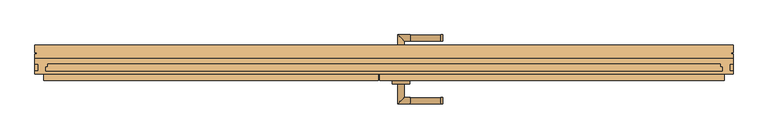
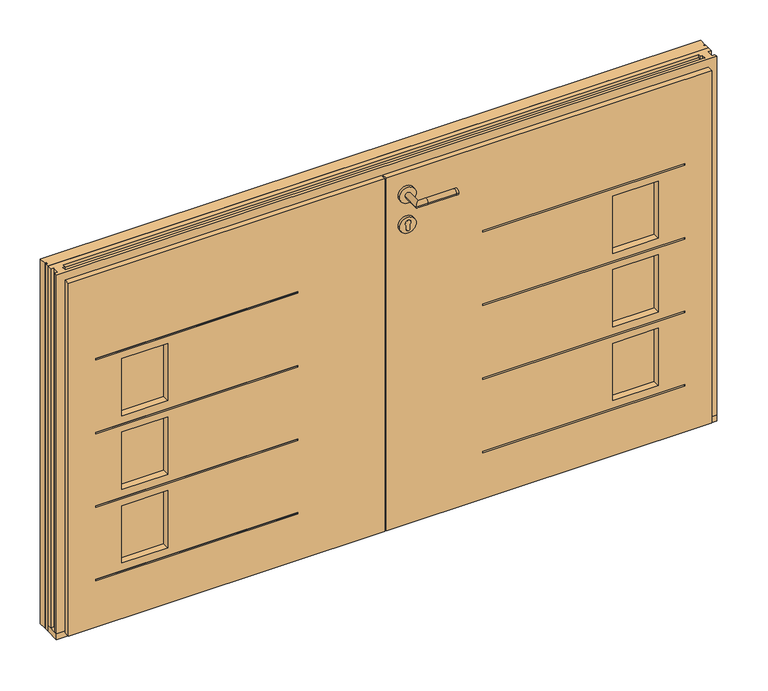
"""IFC4 building model written with IfcOpenShell, lengths in millimetres: door geometry."""

from ifc_helpers import new_model, si_unit, point, frame, frame_2d, origin, origin_with_axes, place, context, project, spatial, polyline, circle_curve, ellipse_curve, trimmed, segment, composite_curve, outline, extrude, faceted_brep, source, transform, mapped, element, save
from ifc_brep_helpers import plane_surface, cylinder_surface, advanced_brep


def door_97be9440(model_context):
    return source(origin(), model_context, "Body", "SolidModel", [
        extrude(outline(polyline([(922.0, -28.0), (922.0, -56.0), (82.0, -56.0), (82.0, -28.0), (922.0, -28.0)])), frame((0.0, 0.0, 108.0), z_axis=(0.0, 0.0, 1.0), x_axis=(1.0, 0.0, 0.0)), (0.0, 0.0, 1.0), 990.2),
        advanced_brep(
        [(60.1308541, -89.0, 1120.0), (41.1308541, -89.0, 1120.0), (41.1308541, -149.0, 1120.0), (60.1308541, -130.0, 1120.0), (176.1308541, -130.0, 1120.0), (176.1308541, -149.0, 1120.0), (170.1308541, -130.0, 1120.0), (170.1308541, -149.0, 1120.0), (79.1308541, -149.0, 1120.0), (79.1308541, -130.0, 1120.0), (170.1308541, -130.5, 1120.0), (170.1308541, -148.5, 1120.0), (79.1308541, -130.5, 1120.0), (79.1308541, -148.5, 1120.0)],
        [
            (0, 1, circle_curve(frame((50.6308541, -89.0, 1120.0), z_axis=(0.0, 1.0, 0.0), x_axis=(-1.0, 0.0, 0.0)), 9.5)),
            (1, 0, circle_curve(frame((50.6308541, -89.0, 1120.0), z_axis=(0.0, 1.0, 0.0), x_axis=(-1.0, 0.0, 0.0)), 9.5)),
            (1, 2),
            (2, 3, ellipse_curve(frame((50.6308541, -139.5, 1120.0), z_axis=(-0.7071067811865475, 0.7071067811865475, 0.0), x_axis=(0.7071067811865474, 0.7071067811865476, 0.0)), 13.4350288, 9.5)),
            (3, 0),
            (3, 2, ellipse_curve(frame((50.6308541, -139.5, 1120.0), z_axis=(-0.7071067811865475, 0.7071067811865475, 0.0), x_axis=(0.7071067811865474, 0.7071067811865476, 0.0)), 13.4350288, 9.5)),
            (4, 5, circle_curve(frame((176.1308541, -139.5, 1120.0), z_axis=(1.0, 0.0, 0.0), x_axis=(0.0, -1.0, 0.0)), 9.5)),
            (5, 4, circle_curve(frame((176.1308541, -139.5, 1120.0), z_axis=(1.0, 0.0, 0.0), x_axis=(0.0, -1.0, 0.0)), 9.5)),
            (4, 6),
            (6, 7, circle_curve(frame((170.1308541, -139.5, 1120.0), z_axis=(1.0, 0.0, 0.0), x_axis=(0.0, -1.0, 0.0)), 9.5)),
            (7, 5),
            (2, 8),
            (8, 9, circle_curve(frame((79.1308541, -139.5, 1120.0), z_axis=(-1.0, 0.0, 0.0), x_axis=(0.0, -1.0, 0.0)), 9.5)),
            (9, 3),
            (9, 8, circle_curve(frame((79.1308541, -139.5, 1120.0), z_axis=(-1.0, 0.0, 0.0), x_axis=(0.0, -1.0, 0.0)), 9.5)),
            (7, 6, circle_curve(frame((170.1308541, -139.5, 1120.0), z_axis=(1.0, 0.0, 0.0), x_axis=(0.0, -1.0, 0.0)), 9.5)),
            (10, 11, circle_curve(frame((170.1308541, -139.5, 1120.0), z_axis=(1.0, 0.0, 0.0), x_axis=(0.0, -1.0, 0.0)), 9.0)),
            (11, 10, circle_curve(frame((170.1308541, -139.5, 1120.0), z_axis=(1.0, 0.0, 0.0), x_axis=(0.0, -1.0, 0.0)), 9.0)),
            (12, 13, circle_curve(frame((79.1308541, -139.5, 1120.0), z_axis=(-1.0, 0.0, 0.0), x_axis=(0.0, -1.0, 0.0)), 9.0)),
            (13, 12, circle_curve(frame((79.1308541, -139.5, 1120.0), z_axis=(-1.0, 0.0, 0.0), x_axis=(0.0, -1.0, 0.0)), 9.0)),
            (10, 12),
            (13, 11),
        ],
        [
            plane_surface(frame((50.6308541, -89.0, 1120.0), z_axis=(0.0, 1.0, 0.0), x_axis=(0.0, 0.0, 1.0))),
            cylinder_surface(frame((50.6308541, -89.0, 1120.0), z_axis=(0.0, 1.0, 0.0), x_axis=(-1.0, 0.0, 0.0)), 9.5),
            plane_surface(frame((176.1308541, -139.5, 1120.0), z_axis=(1.0, 0.0, 0.0), x_axis=(0.0, 0.0, 1.0))),
            cylinder_surface(frame((50.6308541, -139.5, 1120.0), z_axis=(-1.0, 0.0, 0.0), x_axis=(0.0, -1.0, 0.0)), 9.5),
            plane_surface(frame((170.1308541, -149.0, 1120.0), z_axis=(-1.0, 0.0, 0.0), x_axis=(0.0, 0.0, 1.0))),
            plane_surface(frame((79.1308541, -149.0, 1120.0), z_axis=(1.0, 0.0, 0.0), x_axis=(0.0, 0.0, -1.0))),
            cylinder_surface(frame((50.6308541, -139.5, 1120.0), z_axis=(-1.0, 0.0, 0.0), x_axis=(0.0, -1.0, 0.0)), 9.0),
        ],
        [
            (0, [[1, 2]]),
            (1, [[3, 4, 5, -2]]),
            (1, [[-5, 6, -3, -1]]),
            (2, [[7, 8]]),
            (3, [[9, 10, 11, -7]]),
            (3, [[12, 13, 14, -4]]),
            (3, [[-14, 15, -12, -6]]),
            (3, [[-11, 16, -9, -8]]),
            (4, [[-16, -10], [17, 18]]),
            (5, [[-15, -13], [19, 20]]),
            (6, [[21, -20, 22, -17]]),
            (6, [[-22, -19, -21, -18]]),
        ],
    ),
        extrude(outline(composite_curve([segment(trimmed(circle_curve(frame_2d((1019.75, 50.6308541)), 26.0), [point((1019.75, 24.6308541))], [point((1019.75, 76.6308541))], False, "CARTESIAN"), True, "CONTINUOUS"), segment(trimmed(circle_curve(frame_2d((1019.75, 50.6308541)), 26.0), [point((1019.75, 76.6308541))], [point((1019.75, 24.6308541))], False, "CARTESIAN"), True, "CONTINUOUS")], self_intersect=False)), frame((0.0, -89.0, 0.0), z_axis=(0.0, 1.0, 0.0), x_axis=(0.0, 0.0, 1.0)), (0.0, 0.0, 1.0), 10.0),
        extrude(outline(composite_curve([segment(polyline([(1021.404547, 44.8808541), (1008.0, 44.8808541)]), True, "CONTINUOUS"), segment(trimmed(circle_curve(frame_2d((1008.0, 50.6308541)), 5.75), [point((1008.0, 44.8808541))], [point((1008.0, 56.3808541))], False, "CARTESIAN"), True, "CONTINUOUS"), segment(polyline([(1008.0, 56.3808541), (1021.404547, 56.3808541)]), True, "CONTINUOUS"), segment(trimmed(circle_curve(frame_2d((1028.0, 50.6308541)), 8.75), [point((1021.404547, 56.3808541))], [point((1021.404547, 44.8808541))], False, "CARTESIAN"), True, "CONTINUOUS")], self_intersect=False)), frame((0.0, -90.0, 0.0), z_axis=(0.0, 1.0, 0.0), x_axis=(0.0, 0.0, 1.0)), (0.0, 0.0, 1.0), 1.0),
        extrude(outline(composite_curve([segment(trimmed(circle_curve(frame_2d((1120.0, 50.6308541)), 26.0), [point((1120.0, 24.6308541))], [point((1120.0, 76.6308541))], False, "CARTESIAN"), True, "CONTINUOUS"), segment(trimmed(circle_curve(frame_2d((1120.0, 50.6308541)), 26.0), [point((1120.0, 76.6308541))], [point((1120.0, 24.6308541))], False, "CARTESIAN"), True, "CONTINUOUS")], self_intersect=False)), frame((0.0, -89.0, 0.0), z_axis=(0.0, 1.0, 0.0), x_axis=(0.0, 0.0, 1.0)), (0.0, 0.0, 1.0), 10.0),
        advanced_brep(
        [(60.1308541, -2.0, 1120.0), (41.1308541, -2.0, 1120.0), (60.1308541, 39.0, 1120.0), (41.1308541, 58.0, 1120.0), (176.1308541, 39.0, 1120.0), (176.1308541, 58.0, 1120.0), (79.1308541, 39.0, 1120.0), (79.1308541, 58.0, 1120.0), (170.1308541, 58.0, 1120.0), (170.1308541, 39.0, 1120.0), (170.1308541, 39.5, 1120.0), (170.1308541, 57.5, 1120.0), (79.1308541, 39.5, 1120.0), (79.1308541, 57.5, 1120.0)],
        [
            (0, 1, circle_curve(frame((50.6308541, -2.0, 1120.0), z_axis=(0.0, -1.0, 0.0), x_axis=(-1.0, 0.0, 0.0)), 9.5)),
            (1, 0, circle_curve(frame((50.6308541, -2.0, 1120.0), z_axis=(0.0, -1.0, 0.0), x_axis=(-1.0, 0.0, 0.0)), 9.5)),
            (0, 2),
            (2, 3, ellipse_curve(frame((50.6308541, 48.5, 1120.0), z_axis=(-0.7071067811865475, -0.7071067811865475, 0.0), x_axis=(0.7071067811865474, -0.7071067811865476, 0.0)), 13.4350288, 9.5)),
            (3, 1),
            (3, 2, ellipse_curve(frame((50.6308541, 48.5, 1120.0), z_axis=(-0.7071067811865475, -0.7071067811865475, 0.0), x_axis=(0.7071067811865474, -0.7071067811865476, 0.0)), 13.4350288, 9.5)),
            (4, 5, circle_curve(frame((176.1308541, 48.5, 1120.0), z_axis=(1.0, 0.0, 0.0), x_axis=(0.0, 1.0, 0.0)), 9.5)),
            (5, 4, circle_curve(frame((176.1308541, 48.5, 1120.0), z_axis=(1.0, 0.0, 0.0), x_axis=(0.0, 1.0, 0.0)), 9.5)),
            (2, 6),
            (6, 7, circle_curve(frame((79.1308541, 48.5, 1120.0), z_axis=(-1.0, 0.0, 0.0), x_axis=(0.0, 1.0, 0.0)), 9.5)),
            (7, 3),
            (5, 8),
            (8, 9, circle_curve(frame((170.1308541, 48.5, 1120.0), z_axis=(1.0, 0.0, 0.0), x_axis=(0.0, 1.0, 0.0)), 9.5)),
            (9, 4),
            (7, 6, circle_curve(frame((79.1308541, 48.5, 1120.0), z_axis=(-1.0, 0.0, 0.0), x_axis=(0.0, 1.0, 0.0)), 9.5)),
            (9, 8, circle_curve(frame((170.1308541, 48.5, 1120.0), z_axis=(1.0, 0.0, 0.0), x_axis=(0.0, 1.0, 0.0)), 9.5)),
            (10, 11, circle_curve(frame((170.1308541, 48.5, 1120.0), z_axis=(1.0, 0.0, 0.0), x_axis=(0.0, 1.0, 0.0)), 9.0)),
            (11, 10, circle_curve(frame((170.1308541, 48.5, 1120.0), z_axis=(1.0, 0.0, 0.0), x_axis=(0.0, 1.0, 0.0)), 9.0)),
            (12, 13, circle_curve(frame((79.1308541, 48.5, 1120.0), z_axis=(-1.0, 0.0, 0.0), x_axis=(0.0, 1.0, 0.0)), 9.0)),
            (13, 12, circle_curve(frame((79.1308541, 48.5, 1120.0), z_axis=(-1.0, 0.0, 0.0), x_axis=(0.0, 1.0, 0.0)), 9.0)),
            (11, 13),
            (12, 10),
        ],
        [
            plane_surface(frame((50.6308541, -2.0, 1120.0), z_axis=(0.0, -1.0, 0.0), x_axis=(0.0, 0.0, 1.0))),
            cylinder_surface(frame((50.6308541, -2.0, 1120.0), z_axis=(0.0, -1.0, 0.0), x_axis=(-1.0, 0.0, 0.0)), 9.5),
            plane_surface(frame((176.1308541, 48.5, 1120.0), z_axis=(1.0, 0.0, 0.0), x_axis=(0.0, 0.0, 1.0))),
            cylinder_surface(frame((50.6308541, 48.5, 1120.0), z_axis=(-1.0, 0.0, 0.0), x_axis=(0.0, 1.0, 0.0)), 9.5),
            plane_surface(frame((170.1308541, 58.0, 1120.0), z_axis=(-1.0, 0.0, 0.0), x_axis=(0.0, 0.0, 1.0))),
            plane_surface(frame((79.1308541, 58.0, 1120.0), z_axis=(1.0, 0.0, 0.0), x_axis=(0.0, 0.0, -1.0))),
            cylinder_surface(frame((50.6308541, 48.5, 1120.0), z_axis=(-1.0, 0.0, 0.0), x_axis=(0.0, 1.0, 0.0)), 9.0),
        ],
        [
            (0, [[1, 2]]),
            (1, [[-1, 3, 4, 5]]),
            (1, [[-2, -5, 6, -3]]),
            (2, [[7, 8]]),
            (3, [[-4, 9, 10, 11]]),
            (3, [[-8, 12, 13, 14]]),
            (3, [[-6, -11, 15, -9]]),
            (3, [[-7, -14, 16, -12]]),
            (4, [[-13, -16], [17, 18]]),
            (5, [[-10, -15], [19, 20]]),
            (6, [[-18, 21, -19, 22]]),
            (6, [[-17, -22, -20, -21]]),
        ],
    ),
        extrude(outline(composite_curve([segment(trimmed(circle_curve(frame_2d((1019.75, 50.6308541)), 26.0), [point((1019.75, 24.6308541))], [point((1019.75, 76.6308541))], False, "CARTESIAN"), True, "CONTINUOUS"), segment(trimmed(circle_curve(frame_2d((1019.75, 50.6308541)), 26.0), [point((1019.75, 76.6308541))], [point((1019.75, 24.6308541))], False, "CARTESIAN"), True, "CONTINUOUS")], self_intersect=False)), frame((0.0, -12.0, 0.0), z_axis=(0.0, 1.0, 0.0), x_axis=(0.0, 0.0, 1.0)), (0.0, 0.0, 1.0), 10.0),
        extrude(outline(composite_curve([segment(polyline([(1021.404547, 44.8808541), (1008.0, 44.8808541)]), True, "CONTINUOUS"), segment(trimmed(circle_curve(frame_2d((1008.0, 50.6308541)), 5.75), [point((1008.0, 44.8808541))], [point((1008.0, 56.3808541))], False, "CARTESIAN"), True, "CONTINUOUS"), segment(polyline([(1008.0, 56.3808541), (1021.404547, 56.3808541)]), True, "CONTINUOUS"), segment(trimmed(circle_curve(frame_2d((1028.0, 50.6308541)), 8.75), [point((1021.404547, 56.3808541))], [point((1021.404547, 44.8808541))], False, "CARTESIAN"), True, "CONTINUOUS")], self_intersect=False)), frame((0.0, -2.0, 0.0), z_axis=(0.0, 1.0, 0.0), x_axis=(0.0, 0.0, 1.0)), (0.0, 0.0, 1.0), 1.0),
        extrude(outline(composite_curve([segment(trimmed(circle_curve(frame_2d((1120.0, 50.6308541)), 26.0), [point((1120.0, 24.6308541))], [point((1120.0, 76.6308541))], False, "CARTESIAN"), True, "CONTINUOUS"), segment(trimmed(circle_curve(frame_2d((1120.0, 50.6308541)), 26.0), [point((1120.0, 76.6308541))], [point((1120.0, 24.6308541))], False, "CARTESIAN"), True, "CONTINUOUS")], self_intersect=False)), frame((0.0, -12.0, 0.0), z_axis=(0.0, 1.0, 0.0), x_axis=(0.0, 0.0, 1.0)), (0.0, 0.0, 1.0), 10.0),
        faceted_brep([(986.0, -12.0, 1162.2), (986.0, -27.9981764, 1162.2), (986.0, -27.9981764, 44.0), (986.0, -12.0, 44.0), (18.0, -28.0, 1162.2), (18.0, -28.0, 44.0), (703.0, -28.0, 445.0666667), (703.0, -28.0, 636.6333333), (847.0, -28.0, 636.6333333), (847.0, -28.0, 445.0666667), (703.0, -28.0, 199.0), (703.0, -28.0, 390.5666667), (847.0, -28.0, 390.5666667), (847.0, -28.0, 199.0), (703.0, -28.0, 691.1333333), (703.0, -28.0, 882.7), (847.0, -28.0, 882.7), (847.0, -28.0, 691.1333333), (18.0, -12.0, 44.0), (18.0, -12.0, 1162.2), (703.0, -12.0, 445.0666667), (703.0, -12.0, 636.6333333), (847.0, -12.0, 636.6333333), (847.0, -12.0, 445.0666667), (703.0, -12.0, 199.0), (703.0, -12.0, 390.5666667), (847.0, -12.0, 390.5666667), (847.0, -12.0, 199.0), (292.0, -12.0, 665.1333333), (292.0, -12.0, 660.1333333), (930.0, -12.0, 660.1333333), (930.0, -12.0, 665.1333333), (292.0, -12.0, 419.0666667), (292.0, -12.0, 414.0666667), (930.0, -12.0, 414.0666667), (930.0, -12.0, 419.0666667), (292.0, -12.0, 173.0), (292.0, -12.0, 168.0), (930.0, -12.0, 168.0), (930.0, -12.0, 173.0), (703.0, -12.0, 882.7), (703.0, -12.0, 691.1333333), (847.0, -12.0, 691.1333333), (847.0, -12.0, 882.7), (292.0, -12.0, 911.2), (292.0, -12.0, 906.2), (930.0, -12.0, 906.2), (930.0, -12.0, 911.2), (292.0, -21.0185028, 665.1333333), (292.0, -21.0185028, 660.1333333), (930.0, -21.0185028, 660.1333333), (930.0, -21.0185028, 665.1333333), (292.0, -21.0185028, 419.0666667), (292.0, -21.0185028, 414.0666667), (930.0, -21.0185028, 414.0666667), (930.0, -21.0185028, 419.0666667), (292.0, -21.0185028, 173.0), (292.0, -21.0185028, 168.0), (930.0, -21.0185028, 168.0), (930.0, -21.0185028, 173.0), (292.0, -21.0185028, 911.2), (930.0, -21.0185028, 911.2), (930.0, -21.0185028, 906.2), (292.0, -21.0185028, 906.2)], [[[0, 1, 2, 3]], [[2, 1, 4, 5], [6, 7, 8, 9], [10, 11, 12, 13], [14, 15, 16, 17]], [[18, 5, 4, 19]], [[3, 2, 5, 18]], [[6, 20, 21, 7]], [[7, 21, 22, 8]], [[23, 9, 8, 22]], [[20, 6, 9, 23]], [[10, 24, 25, 11]], [[11, 25, 26, 12]], [[27, 13, 12, 26]], [[24, 10, 13, 27]], [[0, 3, 18, 19], [21, 20, 23, 22], [25, 24, 27, 26], [28, 29, 30, 31], [32, 33, 34, 35], [36, 37, 38, 39], [40, 41, 42, 43], [44, 45, 46, 47]], [[48, 49, 29, 28]], [[49, 50, 30, 29]], [[50, 51, 31, 30]], [[52, 53, 33, 32]], [[53, 54, 34, 33]], [[54, 55, 35, 34]], [[55, 52, 32, 35]], [[56, 57, 37, 36]], [[57, 58, 38, 37]], [[58, 59, 39, 38]], [[59, 56, 36, 39]], [[52, 55, 54, 53]], [[57, 56, 59, 58]], [[60, 61, 62, 63]], [[48, 51, 50, 49]], [[1, 0, 19, 4]], [[14, 41, 40, 15]], [[41, 14, 17, 42]], [[42, 17, 16, 43]], [[15, 40, 43, 16]], [[60, 63, 45, 44]], [[63, 62, 46, 45]], [[62, 61, 47, 46]], [[61, 60, 44, 47]], [[51, 48, 28, 31]]]),
        faceted_brep([(1016.0, -60.0, 1192.2), (1016.0, -79.0, 1192.2), (1016.0, -79.0, 14.0), (1016.0, -60.0, 14.0), (-12.0, -79.0, 1192.2), (-12.0, -79.0, 14.0), (292.0, -79.0, 660.1333333), (292.0, -79.0, 665.1333333), (930.0, -79.0, 665.1333333), (930.0, -79.0, 660.1333333), (703.0, -79.0, 636.6333333), (847.0, -79.0, 636.6333333), (847.0, -79.0, 445.0666667), (703.0, -79.0, 445.0666667), (703.0, -79.0, 390.5666667), (847.0, -79.0, 390.5666667), (847.0, -79.0, 199.0), (703.0, -79.0, 199.0), (292.0, -79.0, 414.0666667), (292.0, -79.0, 419.0666667), (930.0, -79.0, 419.0666667), (930.0, -79.0, 414.0666667), (292.0, -79.0, 168.0), (292.0, -79.0, 173.0), (930.0, -79.0, 173.0), (930.0, -79.0, 168.0), (703.0, -79.0, 882.7), (847.0, -79.0, 882.7), (847.0, -79.0, 691.1333333), (703.0, -79.0, 691.1333333), (292.0, -79.0, 906.2), (292.0, -79.0, 911.2), (930.0, -79.0, 911.2), (930.0, -79.0, 906.2), (-12.0, -60.0, 14.0), (-12.0, -60.0, 1192.2), (847.0, -55.9981764, 636.6333333), (703.0, -55.9981764, 636.6333333), (847.0, -56.0, 445.0666667), (703.0, -55.9981764, 445.0666667), (847.0, -55.9981764, 390.5666667), (703.0, -55.9981764, 390.5666667), (847.0, -56.0, 199.0), (703.0, -55.9981764, 199.0), (292.0, -69.5, 660.1333333), (292.0, -69.5, 665.1333333), (930.0, -69.5, 665.1333333), (930.0, -69.5, 660.1333333), (292.0, -69.5, 414.0666667), (292.0, -69.5, 419.0666667), (930.0, -69.5, 419.0666667), (930.0, -69.5, 414.0666667), (292.0, -69.5, 168.0), (292.0, -69.5, 173.0), (930.0, -69.5, 173.0), (930.0, -69.5, 168.0), (922.0, -56.0, 1098.2), (922.0, -56.0, 108.0), (82.0, -56.0, 108.0), (82.0, -56.0, 1098.2), (847.0, -56.0, 882.7), (703.0, -56.0, 882.7), (703.0, -56.0, 691.1333333), (847.0, -56.0, 691.1333333), (922.0, -28.0, 1098.2), (922.0, -28.0, 108.0), (82.0, -28.0, 108.0), (82.0, -28.0, 1098.2), (986.0, -60.0, 44.0), (986.0, -60.0, 1162.2), (18.0, -60.0, 1162.2), (18.0, -60.0, 44.0), (986.0, -28.0, 1162.2), (986.0, -28.0, 44.0), (18.0, -28.0, 44.0), (18.0, -28.0, 1162.2), (292.0, -69.5, 911.2), (292.0, -69.5, 906.2), (930.0, -69.5, 906.2), (930.0, -69.5, 911.2)], [[[0, 1, 2, 3]], [[2, 1, 4, 5], [6, 7, 8, 9], [10, 11, 12, 13], [14, 15, 16, 17], [18, 19, 20, 21], [22, 23, 24, 25], [26, 27, 28, 29], [30, 31, 32, 33]], [[34, 5, 4, 35]], [[3, 2, 5, 34]], [[36, 11, 10, 37]], [[11, 36, 38, 12]], [[39, 13, 12, 38]], [[37, 10, 13, 39]], [[40, 15, 14, 41]], [[15, 40, 42, 16]], [[43, 17, 16, 42]], [[41, 14, 17, 43]], [[44, 45, 7, 6]], [[46, 47, 9, 8]], [[47, 44, 6, 9]], [[48, 49, 19, 18]], [[49, 50, 20, 19]], [[50, 51, 21, 20]], [[51, 48, 18, 21]], [[52, 53, 23, 22]], [[53, 54, 24, 23]], [[54, 55, 25, 24]], [[55, 52, 22, 25]], [[56, 57, 58, 59], [36, 37, 39, 38], [40, 41, 43, 42], [60, 61, 62, 63]], [[56, 64, 65, 57]], [[57, 65, 66, 58]], [[58, 66, 67, 59]], [[0, 3, 34, 35], [68, 69, 70, 71]], [[72, 69, 68, 73]], [[73, 68, 71, 74]], [[72, 73, 74, 75], [65, 64, 67, 66]], [[74, 71, 70, 75]], [[45, 44, 47, 46]], [[49, 48, 51, 50]], [[53, 52, 55, 54]], [[76, 77, 78, 79]], [[1, 0, 35, 4]], [[69, 72, 75, 70]], [[64, 56, 59, 67]], [[60, 27, 26, 61]], [[61, 26, 29, 62]], [[62, 29, 28, 63]], [[27, 60, 63, 28]], [[77, 76, 31, 30]], [[78, 77, 30, 33]], [[79, 78, 33, 32]], [[76, 79, 32, 31]], [[45, 46, 8, 7]]]),
        extrude(outline(polyline([(-922.0, -28.0), (-41.0, -28.0), (-41.0, -56.0), (-922.0, -56.0), (-922.0, -28.0)])), frame((0.0, 0.0, 108.0), z_axis=(0.0, 0.0, 1.0), x_axis=(1.0, 0.0, 0.0)), (0.0, 0.0, 1.0), 990.2),
        faceted_brep([(-17.0, -60.0, 44.0), (-17.0, -60.0, 1162.2), (-17.0, -60.0, 1192.2), (-17.0, -79.0, 1192.2), (-17.0, -79.0, 14.0), (-17.0, -60.0, 14.0), (-1016.0, -60.0, 14.0), (-1016.0, -60.0, 1192.2), (-986.0, -60.0, 1162.2), (-986.0, -60.0, 44.0), (-1016.0, -79.0, 14.0), (-1016.0, -79.0, 1192.2), (-703.0, -79.0, 636.6333333), (-703.0, -79.0, 445.0666667), (-847.0, -79.0, 445.0666667), (-847.0, -79.0, 636.6333333), (-703.0, -79.0, 390.5666667), (-703.0, -79.0, 199.0), (-847.0, -79.0, 199.0), (-847.0, -79.0, 390.5666667), (-930.0, -79.0, 414.0666667), (-930.0, -79.0, 419.0666667), (-292.0, -79.0, 419.0666667), (-292.0, -79.0, 414.0666667), (-930.0, -79.0, 168.0), (-930.0, -79.0, 173.0), (-292.0, -79.0, 173.0), (-292.0, -79.0, 168.0), (-703.0, -79.0, 882.7), (-703.0, -79.0, 691.1333333), (-847.0, -79.0, 691.1333333), (-847.0, -79.0, 882.7), (-930.0, -79.0, 906.2), (-930.0, -79.0, 911.2), (-292.0, -79.0, 911.2), (-292.0, -79.0, 906.2), (-930.0, -79.0, 660.1333333), (-930.0, -79.0, 665.1333333), (-292.0, -79.0, 665.1333333), (-292.0, -79.0, 660.1333333), (-6.0, -60.0, 44.0), (-6.0, -60.0, 1162.2), (-847.0, -56.0, 445.0666667), (-847.0, -55.9981764, 636.6333333), (-703.0, -55.9981764, 445.0666667), (-703.0, -55.9981764, 636.6333333), (-847.0, -56.0, 390.5666667), (-703.0, -55.9981764, 390.5666667), (-847.0, -56.0, 199.0), (-703.0, -55.9981764, 199.0), (-930.0, -74.0, 414.0666667), (-292.0, -74.0, 414.0666667), (-292.0, -74.0, 419.0666667), (-930.0, -74.0, 419.0666667), (-930.0, -74.0, 168.0), (-292.0, -74.0, 168.0), (-292.0, -74.0, 173.0), (-930.0, -74.0, 173.0), (-922.0, -55.9981764, 108.0), (-922.0, -27.9981764, 108.0), (-922.0, -27.9981764, 1098.2), (-922.0, -55.9981764, 1098.2), (-41.0, -55.9981764, 1098.2), (-41.0, -55.9981764, 108.0), (-847.0, -55.9981764, 882.7), (-847.0, -55.9981764, 691.1333333), (-703.0, -55.9981764, 691.1333333), (-703.0, -55.9981764, 882.7), (-41.0, -27.9981764, 108.0), (-41.0, -27.9981764, 1098.2), (-986.0, -27.9981764, 1162.2), (-6.0, -27.9981764, 1162.2), (-6.0, -27.9981764, 44.0), (-986.0, -27.9981764, 44.0), (-292.0, -74.0, 906.2), (-292.0, -74.0, 911.2), (-930.0, -74.0, 911.2), (-930.0, -74.0, 906.2), (-292.0, -74.0, 660.1333333), (-292.0, -74.0, 665.1333333), (-930.0, -74.0, 665.1333333), (-930.0, -74.0, 660.1333333)], [[[0, 1, 2, 3, 4, 5]], [[5, 6, 7, 2, 1, 8, 9, 0]], [[4, 10, 6, 5]], [[4, 3, 11, 10], [12, 13, 14, 15], [16, 17, 18, 19], [20, 21, 22, 23], [24, 25, 26, 27], [28, 29, 30, 31], [32, 33, 34, 35], [36, 37, 38, 39]], [[1, 0, 40, 41]], [[11, 7, 6, 10]], [[15, 14, 42, 43]], [[44, 42, 14, 13]], [[45, 44, 13, 12]], [[16, 19, 46, 47]], [[19, 18, 48, 46]], [[49, 48, 18, 17]], [[47, 49, 17, 16]], [[50, 20, 23, 51]], [[51, 23, 22, 52]], [[52, 22, 21, 53]], [[53, 21, 20, 50]], [[54, 24, 27, 55]], [[55, 27, 26, 56]], [[56, 26, 25, 57]], [[57, 25, 24, 54]], [[58, 59, 60, 61]], [[61, 62, 63, 58], [43, 42, 44, 45], [46, 48, 49, 47], [64, 65, 66, 67]], [[58, 63, 68, 59]], [[68, 63, 62, 69]], [[70, 71, 72, 73], [59, 68, 69, 60]], [[73, 9, 8, 70]], [[73, 72, 40, 0, 9]], [[41, 40, 72, 71]], [[51, 52, 53, 50]], [[55, 56, 57, 54]], [[74, 75, 76, 77]], [[78, 79, 80, 81]], [[60, 69, 62, 61]], [[3, 2, 7, 11]], [[8, 1, 41, 71, 70]], [[28, 31, 64, 67]], [[67, 66, 29, 28]], [[66, 65, 30, 29]], [[31, 30, 65, 64]], [[12, 15, 43, 45]], [[77, 32, 35, 74]], [[76, 33, 32, 77]], [[75, 34, 33, 76]], [[74, 35, 34, 75]], [[81, 36, 39, 78]], [[80, 37, 36, 81]], [[79, 38, 37, 80]], [[78, 39, 38, 79]]]),
        extrude(outline(polyline([(18.0, -12.0), (18.0, -28.0), (-41.0, -28.0), (-41.0, -12.0), (18.0, -12.0)])), frame((0.0, 0.0, 44.0), z_axis=(0.0, 0.0, 1.0), x_axis=(1.0, 0.0, 0.0)), (0.0, 0.0, 1.0), 1118.2),
        faceted_brep([(23.5, -12.0, 49.0), (-22.5, -12.0, 49.0), (-20.5, -4.0, 49.0), (21.5, -4.0, 49.0), (23.5, -12.0, 1157.7), (21.5, -4.0, 1157.7), (-20.5, -4.0, 1157.7), (-22.5, -12.0, 1157.7)], [[[0, 1, 2, 3]], [[4, 0, 3, 5]], [[5, 3, 2, 6]], [[6, 2, 1, 7]], [[7, 1, 0, 4]], [[4, 5, 6, 7]]]),
        faceted_brep([(-41.0, -12.0, 44.0), (-41.0, -12.0, 1162.2), (-41.0, -27.9981764, 1162.2), (-41.0, -27.9981764, 44.0), (-986.0, -27.9981764, 44.0), (-986.0, -12.0, 44.0), (-986.0, -27.9981764, 1162.2), (-703.0, -27.9981764, 636.6333333), (-703.0, -27.9981764, 445.0666667), (-847.0, -27.9981764, 445.0666667), (-847.0, -27.9981764, 636.6333333), (-703.0, -27.9981764, 390.5666667), (-703.0, -27.9981764, 199.0), (-847.0, -27.9981764, 199.0), (-847.0, -27.9981764, 390.5666667), (-703.0, -27.9981764, 882.7), (-703.0, -27.9981764, 691.1333333), (-847.0, -27.9981764, 691.1333333), (-847.0, -27.9981764, 882.7), (-986.0, -12.0, 1162.2), (-847.0, -12.0, 636.6333333), (-847.0, -12.0, 445.0666667), (-703.0, -12.0, 445.0666667), (-703.0, -12.0, 636.6333333), (-847.0, -12.0, 390.5666667), (-847.0, -12.0, 199.0), (-703.0, -12.0, 199.0), (-703.0, -12.0, 390.5666667), (-930.0, -12.0, 419.0666667), (-930.0, -12.0, 414.0666667), (-292.0, -12.0, 414.0666667), (-292.0, -12.0, 419.0666667), (-930.0, -12.0, 173.0), (-930.0, -12.0, 168.0), (-292.0, -12.0, 168.0), (-292.0, -12.0, 173.0), (-847.0, -12.0, 882.7), (-847.0, -12.0, 691.1333333), (-703.0, -12.0, 691.1333333), (-703.0, -12.0, 882.7), (-930.0, -12.0, 665.1333333), (-930.0, -12.0, 660.1333333), (-292.0, -12.0, 660.1333333), (-292.0, -12.0, 665.1333333), (-930.0, -12.0, 906.2), (-292.0, -12.0, 906.2), (-292.0, -12.0, 911.2), (-930.0, -12.0, 911.2), (-930.0, -17.0, 419.0666667), (-292.0, -17.0, 419.0666667), (-292.0, -17.0, 414.0666667), (-930.0, -17.0, 414.0666667), (-930.0, -17.0, 173.0), (-292.0, -17.0, 173.0), (-292.0, -17.0, 168.0), (-930.0, -17.0, 168.0), (-930.0, -17.0, 665.1333333), (-292.0, -17.0, 665.1333333), (-292.0, -17.0, 660.1333333), (-930.0, -17.0, 660.1333333), (-930.0, -17.0, 906.2), (-930.0, -17.0, 911.2), (-292.0, -17.0, 911.2), (-292.0, -17.0, 906.2)], [[[0, 1, 2, 3]], [[3, 4, 5, 0]], [[3, 2, 6, 4], [7, 8, 9, 10], [11, 12, 13, 14], [15, 16, 17, 18]], [[1, 0, 5, 19], [20, 21, 22, 23], [24, 25, 26, 27], [28, 29, 30, 31], [32, 33, 34, 35], [36, 37, 38, 39], [40, 41, 42, 43], [44, 45, 46, 47]], [[5, 4, 6, 19]], [[11, 14, 24, 27]], [[27, 26, 12, 11]], [[26, 25, 13, 12]], [[14, 13, 25, 24]], [[23, 22, 8, 7]], [[22, 21, 9, 8]], [[10, 9, 21, 20]], [[48, 28, 31, 49]], [[49, 31, 30, 50]], [[50, 30, 29, 51]], [[51, 29, 28, 48]], [[52, 32, 35, 53]], [[53, 35, 34, 54]], [[54, 34, 33, 55]], [[55, 33, 32, 52]], [[48, 49, 50, 51]], [[52, 53, 54, 55]], [[56, 57, 58, 59]], [[60, 61, 62, 63]], [[1, 19, 6, 2]], [[7, 10, 20, 23]], [[15, 18, 36, 39]], [[39, 38, 16, 15]], [[38, 37, 17, 16]], [[18, 17, 37, 36]], [[56, 40, 43, 57]], [[57, 43, 42, 58]], [[58, 42, 41, 59]], [[59, 41, 40, 56]], [[60, 44, 47, 61]], [[61, 47, 46, 62]], [[62, 46, 45, 63]], [[63, 45, 44, 60]]]),
        faceted_brep([(1004.0, 27.4665116, 0.0), (1043.0, 27.4665116, 0.0), (1043.0, 5.0, 0.0), (1038.0, 5.0, 0.0), (1038.0, 0.0, 0.0), (1043.0, 0.0, 0.0), (1043.0, -12.0, 0.0), (981.5, -12.0, 0.0), (981.5, -4.0, 0.0), (1004.0, -4.0, 0.0), (-1043.0, 0.0, 0.0), (-1038.0, 0.0, 0.0), (-1038.0, 5.0, 0.0), (-1043.0, 5.0, 0.0), (-1043.0, 27.4665116, 0.0), (-1004.0, 27.4665116, 0.0), (-1004.0, -4.0, 0.0), (-981.5, -4.0, 0.0), (-981.5, -12.0, 0.0), (-1043.0, -12.0, 0.0), (1004.0, -4.0, 1180.2), (1004.0, 27.4665116, 1180.2), (981.5, -12.0, 1157.7), (981.5, -4.0, 1157.7), (-1004.0, 27.4665116, 1180.2), (-1004.0, -4.0, 1180.2), (-981.5, -4.0, 1157.7), (-981.5, -12.0, 1157.7), (-1043.0, -12.0, 1219.2), (-1043.0, 0.0, 1219.2), (-1043.0, 5.0, 1219.2), (-1043.0, 27.4665116, 1219.2), (-1038.0, 5.0, 1219.2), (-1038.0, 0.0, 1219.2), (1043.0, 0.0, 1219.2), (1043.0, -12.0, 1219.2), (1038.0, 0.0, 1219.2), (1038.0, 5.0, 1219.2), (1043.0, 5.0, 1219.2), (1043.0, 27.4665116, 1219.2)], [[[0, 1, 2, 3, 4, 5, 6, 7, 8, 9]], [[10, 11, 12, 13, 14, 15, 16, 17, 18, 19]], [[0, 9, 20, 21]], [[8, 7, 22, 23]], [[24, 21, 20, 25]], [[26, 23, 22, 27]], [[18, 17, 26, 27]], [[25, 16, 15, 24]], [[28, 29, 10, 19]], [[30, 31, 14, 13]], [[32, 30, 13, 12]], [[33, 32, 12, 11]], [[29, 33, 11, 10]], [[34, 35, 6, 5]], [[36, 34, 5, 4]], [[37, 36, 4, 3]], [[38, 37, 3, 2]], [[39, 38, 2, 1]], [[39, 1, 0, 21, 24, 15, 14, 31]], [[9, 8, 23, 26, 17, 16, 25, 20]], [[27, 22, 7, 6, 35, 28, 19, 18]], [[39, 31, 30, 32, 33, 29, 28, 35, 34, 36, 37, 38]]]),
        faceted_brep([(1010.0, -60.0, 20.0), (1010.0, -38.0, 20.0), (1004.0, -38.0, 20.0), (1004.0, -12.0, 20.0), (1043.0, -12.0, 20.0), (1043.0, -29.0, 20.0), (1033.0, -29.0, 20.0), (1033.0, -50.0, 20.0), (1043.0, -50.0, 20.0), (1043.0, -60.0, 20.0), (-1010.0, -60.0, 20.0), (-1043.0, -60.0, 20.0), (-1043.0, -50.0, 20.0), (-1033.0, -50.0, 20.0), (-1033.0, -29.0, 20.0), (-1043.0, -29.0, 20.0), (-1043.0, -12.0, 20.0), (-1004.0, -12.0, 20.0), (-1004.0, -38.0, 20.0), (-1010.0, -38.0, 20.0), (1043.0, -60.0, 1219.2), (-1043.0, -60.0, 1219.2), (-1010.0, -60.0, 1186.2), (1010.0, -60.0, 1186.2), (1043.0, -50.0, 1219.2), (1033.0, -50.0, 1219.2), (1033.0, -29.0, 1219.2), (1004.0, -12.0, 1186.2), (-1004.0, -12.0, 1186.2), (-1043.0, -12.0, 1219.2), (1043.0, -12.0, 1219.2), (1004.0, -38.0, 1186.2), (1004.0, -38.0, 1219.2), (1004.0, -29.0, 1219.2), (1004.0, -29.0, 1209.2), (1004.0, -38.0, 1209.2), (1010.0, -38.0, 1186.2), (1010.0, -38.0, 1219.2), (1010.0, -38.0, 1209.2), (1010.0, -50.0, 1219.2), (1010.0, -50.0, 1209.2), (-1010.0, -38.0, 1186.2), (-1010.0, -38.0, 1219.2), (-1010.0, -50.0, 1219.2), (-1010.0, -50.0, 1209.2), (-1010.0, -38.0, 1209.2), (-1004.0, -38.0, 1186.2), (-1004.0, -38.0, 1219.2), (-1004.0, -38.0, 1209.2), (-1004.0, -29.0, 1219.2), (-1004.0, -29.0, 1209.2), (-1043.0, -29.0, 1219.2), (1043.0, -29.0, 1219.2), (-1033.0, -29.0, 1219.2), (-1033.0, -50.0, 1219.2), (-1043.0, -50.0, 1219.2)], [[[0, 1, 2, 3, 4, 5, 6, 7, 8, 9]], [[10, 11, 12, 13, 14, 15, 16, 17, 18, 19]], [[20, 21, 11, 10, 22, 23, 0, 9]], [[24, 20, 9, 8]], [[25, 24, 8, 7]], [[26, 25, 7, 6]], [[4, 3, 27, 28, 17, 16, 29, 30]], [[3, 2, 31, 27]], [[32, 33, 34, 35]], [[2, 1, 36, 31]], [[37, 32, 35, 38]], [[1, 0, 23, 36]], [[39, 37, 38, 40]], [[10, 19, 41, 22]], [[42, 43, 44, 45]], [[19, 18, 46, 41]], [[47, 42, 45, 48]], [[18, 17, 28, 46]], [[49, 47, 48, 50]], [[51, 29, 16, 15]], [[43, 39, 40, 44]], [[44, 40, 38, 35, 34, 50, 48, 45]], [[33, 49, 50, 34]], [[23, 22, 41, 46, 28, 27, 31, 36]], [[20, 24, 25, 26, 52, 30, 29, 51, 53, 54, 55, 21], [37, 39, 43, 42, 47, 49, 33, 32]], [[30, 52, 5, 4]], [[21, 55, 12, 11]], [[52, 26, 6, 5]], [[53, 51, 15, 14]], [[54, 53, 14, 13]], [[55, 54, 13, 12]]]),
        extrude(outline(polyline([(-9.4223795, 35.1), (-6.0676205, 35.1), (-7.04, 32.9), (-7.04, 20.0), (-8.45, 20.0), (-8.45, 32.9), (-9.4223795, 35.1)])), frame((-981.5, 0.0, 0.0), z_axis=(1.0, 0.0, 0.0), x_axis=(0.0, 1.0, 0.0)), (0.0, 0.0, 1.0), 1963.0),
        extrude(outline(polyline([(-1004.0, -12.0), (-1004.0, 5.0), (1004.0, 5.0), (1004.0, -12.0), (-1004.0, -12.0)])), origin_with_axes(), (0.0, 0.0, 1.0), 20.0),
        extrude(outline(polyline([(-1043.0, -60.0), (-1043.0, -12.0), (1043.0, -12.0), (1043.0, -60.0), (-1043.0, -60.0)])), origin_with_axes(), (0.0, 0.0, 1.0), 20.0),
        extrude(outline(polyline([(-12.0, 54.3693722), (6.11, 51.18), (6.11, 47.11), (4.51, 47.11), (4.51, 49.84), (-10.4, 52.4658167), (-10.4, 40.3), (-3.6, 40.3), (-3.6, 35.1), (-12.0, 35.1), (-12.0, 54.3693722)])), frame((-981.5, 0.0, 0.0), z_axis=(1.0, 0.0, 0.0), x_axis=(0.0, 1.0, 0.0)), (0.0, 0.0, 1.0), 1963.0),
    ])


if __name__ == "__main__":
    model = new_model("IFC4")
    model_context = context("Model", 3, world=origin())
    ifc_project = project(units=[si_unit("LENGTHUNIT", "METRE", prefix="MILLI")], contexts=[model_context])
    site = spatial("IfcSite", under=ifc_project)
    building = spatial("IfcBuilding", under=site)
    placement = place(None, origin())
    door_shape = door_97be9440(model_context)
    element("IfcDoor", 1, at=placement, inside=building, context=model_context, shape_type="MappedRepresentation", body=[
        mapped(door_shape, transform((0.0, 0.0, 0.0), x_axis=(1.0, 0.0, 0.0), y_axis=(0.0, 1.0, 0.0), z_axis=(0.0, 0.0, 1.0))),
    ])
    save(model, "model.ifc")

# Revit data of these elements
# Type
#   Type Mark = "40"
#   Version Revit = "Revit 2017"
#   Uniformat II description = "Double door"
#   Uniformat CSI = "B2030"
#   URL = "https://www.fenetremeo.com/porte-entree"
#   Type de pose = "Tunnel"
#   Référence modèle = "MeO-PE-BALADE-2vtx"
#   Pose vitrage = "Vitrage collé"
#   Keynote = "MeO-PE-BALADE-2vtx"
#   Neuf / Réno = "Rénovation"
#   Model = "Porte double BALADE"
#   Matériaux = "Aluminium / bois"
#   IFC version = "IFC 2x3 Coordination 2.0"
#   IFC classification = "Door"
#   Fiches produits = "https://www.fenetremeo.com/porte-entree"
#   Famille de produit = "Porte"
#   Manufacturer = "MéO"
#   FILE_NAME = "2021-07-MeO-PE-BALADE-2vtx"
#   Design = "Modélisation non contractuelle"
#   Description = "Porte 2 vantaux égaux"
#   Contraintes largeur porte = "700 < Largeur < 1200"
#   Contraintes hauteur porte = "1953 < Hauteur < 2500"
#   Contraintes hauteur poignée porte = "900 <Hauteur poignée < 1300"
#   Analytic Construction = "<Aucun>"
#   Coefficient thermique Ud = "0.72 / 0.75 Ud"
#   BIMobject main category = "Exterior carpentry"
#   Avis technique = "https://www.fcba.fr/wp-content/uploads/2020/10/rc_nf297.pdf"
#   Surface = 7854.671916 ft
#   Pose tunnel = 0.032808 ft
#   Longueur de traverse haute 33,43,53,63,73,83 = 0.108268 ft
#   Largeur zone 2 = 3.28084 ft
#   Largeur zone 1 = 3.28084 ft
#   Largeur du dormant 33,43,53,63,73,83 = 0.108268 ft
#   Rough Width = 6.843832 ft
#   Hauteur poignée = 3.608924 ft
#   Hauteur dormant = 4 ft
#   Rough Height = 4 ft
#   HT ouvrant = 3.826115 ft
#   Height = 3.888451 ft
#   Width = 6.627297 ft
#   Doublage 75,105,125,145,165,185,205 = 0.286964 ft
#   Message Hors abaques = yes
#   Hors abaques = yes
#   Vitrage = Verre
#   Couleur poignée = Acier inoxydable AISI 304
#   Choix du modèle = element 399773
#   Function = (empty or 0)
#   Wall Closure = (empty or 0)
# Element 1 (IfcDoor)
#   Materials on its faces: "Acier inoxydable AISI 304", "Verre", "Aluminium"
# Materials
#   "Verre": class "Verre", colour RGB 92 99 177, transparency 0.7, Description = "Verre sodocalcique", Cost = 0
#   "Acier inoxydable AISI 304": colour RGB 120 120 120, transparency 0, Description = "Stainless Steel 18/8", Cost = 0
#   "Aluminium": class "Metal", colour RGB 247 247 247, transparency 0, Description = "Aluminium 6061", Cost = 0
